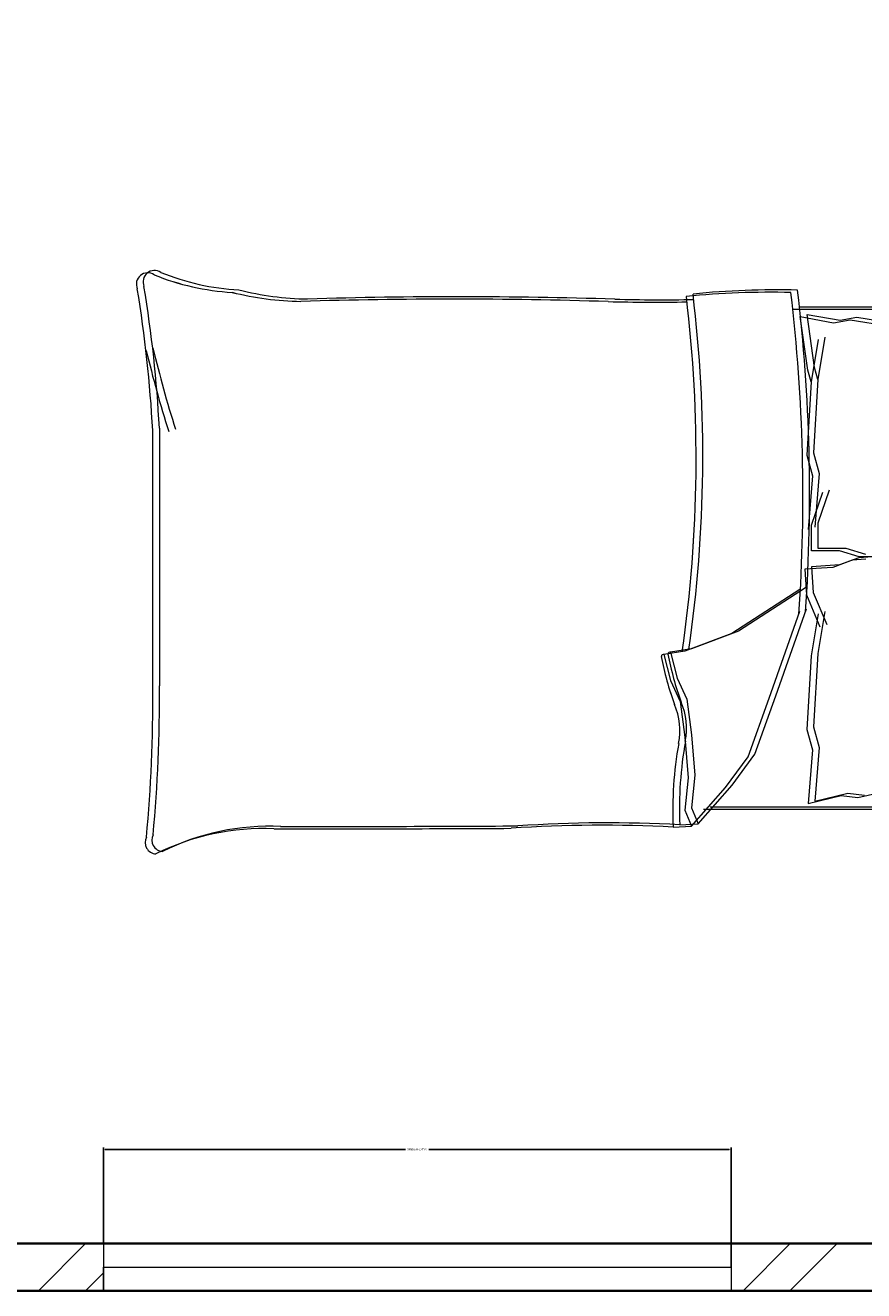
# Model space of a CAD drawing. Units: inches. Extents: x 2120 to 4013, y 1390 to 3019.
# Tile 11 of 59: x 2537 to 2617, y 1582 to 1702. Entities that reach past the tile are written whole.
import ezdxf

# ---------------------------------------------------------------- set-up
doc = ezdxf.new("R2010")
doc.units = ezdxf.units.IN
for name, color, linetype, lineweight in [('A-ANNO-DIMS', 2, 'Continuous', 18), ('A-FURN', 8, 'Continuous', 13), ('A-GLAZ', 4, 'Continuous', 18), ('A-WALL', 7, 'Continuous', 35), ('A-WALL-PATT', 252, 'Continuous', 13)]:
    doc.layers.add(name, color=color, linetype=linetype, lineweight=lineweight)
doc.styles.get("Standard").update_dxf_attribs({"font": 'arial.ttf'})
doc.dimstyles.get("Standard").update_dxf_attribs({"dimtxt": 0.18, "dimasz": 0.18, "dimexe": 0.18, "dimexo": 0.0625, "dimgap": 0.09, "dimtad": 0, "dimtih": 1, "dimtoh": 1, "dimdec": 4, "dimzin": 0, "dimdsep": 46, "dimtxsty": 'Standard', "dimcen": 0.09, "dimadec": 0, "dimazin": 0, "dimtfac": 1, "dimtdec": 4, "dimtofl": 0, "dimtmove": 0, "dimatfit": 3, "dimfxl": 1, "dimtolj": 1, "dimtzin": 0, "dimarcsym": 0})

# ---------------------------------------------------------------- blocks, each defined once
blk = doc.blocks.new('BED-DOUBLE-PLAN')
for p, q in [((3.48, 63.34), (3.48, 81.45)), ((51.27, 81.45), (51.27, 54.84)), ((3.7, 62.7), (3.7, 80.81)), ((51.5, 80.81), (51.5, 54.2)), ((50.34, 68.98), (49.54, 72.55)), ((4.47, 68.88), (5.05, 72.49)), ((4.7, 68.24), (5.28, 71.85)), ((27.36, 70.37), (27.44, 69.07)), ((27.37, 70.41), (27.37, 69.1)), ((27.14, 69.74), (26.56, 67.86)), ((27.37, 69.1), (26.79, 67.23)), ((27.44, 69.07), (28.13, 67.23)), ((27.58, 69.73), (27.67, 68.43)), ((49.92, 68.01), (50.11, 69.62)), ((50.15, 67.37), (50.34, 68.98)), ((4.76, 67.29), (4.47, 68.88)), ((4.99, 66.65), (4.7, 68.24)), ((26.56, 67.86), (26.56, 65.18)), ((27.67, 68.43), (28.36, 66.59)), ((50.7, 64.87), (49.92, 68.01)), ((4.19, 64.11), (4.76, 67.29)), ((4.41, 63.47), (4.99, 66.65)), ((26.79, 67.23), (26.79, 64.54)), ((28.13, 67.23), (28.3, 64.55)), ((28.36, 66.59), (28.53, 63.91)), ((50.93, 64.23), (50.15, 67.37)), ((6.38, 65.82), (10.42, 65.15)), ((24.1, 65.18), (20.96, 66.27)), ((24.33, 64.54), (21.19, 65.63)), ((30.75, 64.71), (33.82, 65.99)), ((30.98, 64.07), (34.05, 65.35)), ((32.57, 65.82), (36.6, 65.15)), ((9.28, 64.83), (4.19, 64.11)), ((9.51, 64.19), (4.41, 63.47)), ((6.61, 65.18), (10.64, 64.51)), ((10.42, 65.15), (9.28, 64.83)), ((10.64, 64.51), (9.51, 64.19)), ((10.42, 65.15), (17.43, 64.72)), ((10.64, 64.51), (17.65, 64.08)), ((17.43, 64.72), (19.39, 65.28)), ((17.65, 64.08), (19.61, 64.64)), ((19.39, 65.28), (24.52, 64.87)), ((19.61, 64.64), (24.75, 64.23)), ((26.56, 65.18), (24.1, 65.18)), ((26.79, 64.54), (24.33, 64.54)), ((28.3, 64.55), (30.75, 64.71)), ((32.79, 65.18), (36.83, 64.51)), ((36.6, 65.15), (43.61, 64.72)), ((36.83, 64.51), (43.84, 64.08)), ((43.61, 64.72), (45.57, 65.28)), ((43.84, 64.08), (45.8, 64.64)), ((45.57, 65.28), (50.7, 64.87)), ((45.8, 64.64), (50.93, 64.23)), ((28.53, 63.91), (30.98, 64.07)), ((30.26, 64.06), (34.45, 57.57)), ((30.49, 63.42), (34.68, 56.93)), ((40.65, 61.13), (32.31, 64.06)), ((40.87, 60.49), (32.54, 63.42)), ((46.22, 59.12), (40.65, 61.13)), ((46.45, 58.48), (40.87, 60.49)), ((49.16, 56.95), (46.22, 59.12)), ((49.39, 56.31), (46.45, 58.48)), ((34.45, 57.57), (36.15, 53.08)), ((34.68, 56.93), (36.38, 52.44)), ((52.87, 53.7), (49.16, 56.95)), ((53.1, 53.06), (49.39, 56.31)), ((44.36, 53.08), (48.23, 53.39)), ((48.23, 53.39), (51.33, 53.08)), ((51.33, 53.08), (52.87, 53.7)), ((52.95, 51.96), (52.87, 53.7, 3.87)), ((36.15, 53.08), (36.46, 51.07)), ((36.38, 52.44), (36.69, 50.43)), ((38.94, 51.69), (40.96, 52.62)), ((40.96, 52.62), (44.36, 53.08)), ((41.18, 51.98), (44.59, 52.44)), ((44.59, 52.44), (48.46, 52.75)), ((48.46, 52.75), (51.56, 52.44)), ((51.56, 52.44), (53.1, 53.06)), ((53.18, 51.32), (53.1, 53.06, 3.87)), ((36.46, 51.07), (38.94, 51.69)), ((36.69, 50.43), (39.17, 51.05)), ((39.17, 51.05), (41.18, 51.98)), ((15.06, 2.2), (39.68, 2.2)), ((15.29, 1.56), (39.91, 1.56))]:
    blk.add_line(p, q)
for centre, radius, start, end in [((21.36, -100.61), 164.97, 86.0865, 96.7821), ((85.16, 61.35), 83.31, 178.7218, 185.604), ((21.59, -101.25), 164.97, 86.0865, 96.7821), ((85.39, 60.71), 83.31, 178.7218, 185.604), ((17.76, -74.87), 129.02, 81.7845, 96.9006), ((17.99, -75.51), 129.02, 81.7845, 96.9006), ((-167.31, 50.27), 170.11, 358.4762, 1.0082), ((-167.08, 49.63), 170.11, 358.4762, 1.0082), ((31.16, 79.96), 29.65, 280.6617, 289.8806), ((43.74, 46.38), 6.22, 78.6608, 113.7384), ((51.33, 88.1), 36.18, 259.8763, 272.5657), ((36.64, 51.01), 0.185, 160.2464, 271.1377), ((31.38, 79.32), 29.65, 280.6617, 289.8806), ((43.97, 45.74), 6.22, 78.6608, 113.7384), ((51.56, 87.46), 36.18, 259.8763, 272.5657), ((182.27, 45.13), 129.5, 176.9791, 183.8365), ((182.5, 44.49), 129.5, 176.9791, 183.8365), ((36.87, 50.37), 0.185, 160.2464, 271.1377), ((484.82, 30.83), 482.31, 178.2277, 181.7185), ((485.05, 30.19), 482.31, 178.2277, 181.7185), ((-4508.74, 13.62), 4561.86, 0.00217, 0.28689), ((-4508.51, 12.99), 4561.86, 0.00217, 0.28689), ((-26.9, 16.93), 29.63, 346.0648, 358.9113), ((-26.67, 16.29), 29.63, 346.0648, 358.9113), ((76.16, 12.78), 23.07, 177.4714, 206.4681), ((76.39, 12.14), 23.07, 177.4714, 206.4681), ((-21.66, 11.17), 23.56, 337.9751, 356.652), ((-21.43, 10.53), 23.56, 337.9751, 356.652), ((-17.22, 105.16), 106.46, 283.3832, 287.7053), ((-16.99, 104.52), 106.46, 283.3832, 287.7053), ((54.41, 2.58), 1.1, 242.6588, 356.02), ((1.09, 1.73), 1.09, 146.1736, 293.4781), ((1.32, 1.09), 1.09, 146.1736, 293.4781), ((21.43, -119.39), 121.76, 92.9958, 99.4091), ((21.66, -120.03), 121.76, 92.9958, 99.4091), ((41.15, -130.83), 133.04, 84.4998, 90.6351), ((41.38, -131.47), 133.04, 84.4998, 90.6351), ((54.64, 1.94), 1.1, 242.6588, 356.02)]:
    blk.add_arc(centre, radius, start, end)
blk = doc.blocks.new('WIN-PLAN-60IN-05')
for p, q in [((0, 4.5), (0, 0)), ((60, 2.25), (60, 4.5)), ((60, 4.5), (60, 4.5)), ((60, 4.5), (60, 0)), ((0, 0), (0, 2.25)), ((0, 2.25), (60, 2.25))]:
    blk.add_line(p, q)
blk = doc.blocks.new('*D191')
at = {"layer": 'A-ANNO-DIMS', "color": 0, "lineweight": -2, "transparency": 16777216}
for p, q in [((2544.14, 1586.09), (2544.14, 1595.21)), ((2544.32, 1595.03), (2573.02, 1595.03)), ((2603.96, 1595.03), (2575.25, 1595.03)), ((2604.14, 1586.09), (2604.14, 1595.21))]:
    blk.add_line(p, q, dxfattribs=at)
at = {"layer": 'A-ANNO-DIMS', "color": 0, "transparency": 16777216}
for points in [[(2544.32, 1595.06), (2544.32, 1595), (2544.14, 1595.03)], [(2603.96, 1595.06), (2603.96, 1595), (2604.14, 1595.03)]]:
    blk.add_solid(points, dxfattribs=at)
at = {"layer": 'Defpoints', "color": 0, "transparency": 16777216}
for p in [(2604.14, 1595.03), (2544.14, 1586.03), (2604.14, 1586.03)]:
    blk.add_point(p, dxfattribs=at)
at = {"layer": 'A-ANNO-DIMS', "color": 0, "transparency": 16777216, "insert": (2574.14, 1595.03), "char_height": 0.18, "attachment_point": 5}
blk.add_mtext('\\A1;WINDOW 60 TYP.', dxfattribs=at)
blk = doc.blocks.new('*D192')
at = {"layer": 'A-ANNO-DIMS', "color": 0, "lineweight": -2, "transparency": 16777216}
for p, q in [((2544.07, 1586.03), (2534.96, 1586.03)), ((2535.14, 1585.85), (2535.14, 1583.96)), ((2535.14, 1581.71), (2535.14, 1583.6)), ((2544.07, 1581.53), (2534.96, 1581.53))]:
    blk.add_line(p, q, dxfattribs=at)
at = {"layer": 'A-ANNO-DIMS', "color": 0, "transparency": 16777216}
for points in [[(2535.11, 1585.85), (2535.17, 1585.85), (2535.14, 1586.03)], [(2535.11, 1581.71), (2535.17, 1581.71), (2535.14, 1581.53)]]:
    blk.add_solid(points, dxfattribs=at)
at = {"layer": 'Defpoints', "color": 0, "transparency": 16777216}
for p in [(2535.14, 1586.03), (2544.14, 1586.03), (2544.14, 1581.53)]:
    blk.add_point(p, dxfattribs=at)
at = {"layer": 'A-ANNO-DIMS', "color": 0, "transparency": 16777216, "insert": (2535.14, 1583.78), "char_height": 0.18, "attachment_point": 5}
blk.add_mtext('\\A1;5 TYP.', dxfattribs=at)

msp = doc.modelspace()

# ---------------------------------------------------------------- hatches: boundary and pattern name
at = {"layer": 'A-WALL-PATT'}
h = msp.add_hatch(dxfattribs=at)
h.set_pattern_fill('ANSI32', color=256)
h.paths.add_polyline_path([(2271.7331, 2343.531), (2283.3788, 2343.531), (2283.3788, 2348.031), (2283.3788, 2352.5306), (2262.7331, 2352.5306), (2262.7331, 2182.638), (2267.2331, 2182.638), (2271.7331, 2182.638), (2271.7331, 2219.031), (2391.7331, 2219.031), (2391.7331, 2214.189), (2393.9831, 2214.189), (2396.2331, 2214.189), (2396.2331, 2219.031), (2420.2331, 2219.031), (2420.2331, 2225.7535), (2417.2197, 2225.7535), (2415.7331, 2225.7535), (2415.7331, 2223.5306), (2271.7331, 2223.5306)])
h.paths.add_polyline_path([(2380.0942, 2352.5306), (2343.3788, 2352.5306), (2343.3788, 2343.531), (2363.2331, 2343.531), (2363.2331, 2288.8489), (2365.4831, 2288.8489), (2367.7331, 2288.8489), (2367.7331, 2343.531), (2380.0942, 2343.531)], flags=17)
h.paths.add_polyline_path([(2432.4339, 2352.5306), (2404.0943, 2352.5306), (2404.0943, 2343.531), (2415.7331, 2343.531), (2415.7331, 2264.0306), (2367.7331, 2264.0306), (2367.7331, 2266.4872), (2363.2331, 2266.4872), (2363.2331, 2259.531), (2367.7331, 2259.531), (2415.7331, 2259.531), (2415.7331, 2255.0658), (2420.2331, 2255.0658), (2420.2331, 2259.531), (2424.5717, 2259.531), (2424.5717, 2261.781), (2424.5717, 2264.0306), (2420.2331, 2264.0306), (2420.2331, 2343.531), (2432.4339, 2343.531)])
h.paths.add_polyline_path([(2508.9115, 2352.5306), (2456.4339, 2352.5306), (2456.4339, 2343.531), (2468.2331, 2343.531), (2468.2331, 2264.0306), (2448.0487, 2264.0306), (2448.0487, 2259.531), (2468.2331, 2259.531), (2468.2331, 2255.5496), (2472.7331, 2255.5496), (2472.7331, 2343.531), (2508.9115, 2343.531)])
h.paths.add_polyline_path([(2637.7331, 2352.5306), (2544.9116, 2352.5306), (2544.9116, 2343.531), (2589.7331, 2343.531), (2633.2331, 2343.531), (2637.7331, 2343.531)])
h.paths.add_polyline_path([(2594.2331, 2343.5306), (2589.7331, 2343.5306), (2589.7331, 2259.5306), (2589.7331, 2252.4915), (2591.9831, 2252.4915), (2594.2331, 2252.4915)])
h.paths.add_polyline_path([(2637.7331, 2223.5306), (2594.2331, 2223.5306), (2594.2331, 2230.1988), (2591.9831, 2230.1988), (2589.7331, 2230.1988), (2589.7331, 2223.5306), (2472.7331, 2223.5306), (2468.2331, 2223.5306), (2468.2331, 2219.031), (2628.7331, 2219.031), (2628.7331, 2138.031), (2637.7331, 2138.031)])
h.paths.add_polyline_path([(3822.6535, 2458.4402), (3874.9468, 2458.4402), (3874.9468, 2476.9866), (3822.6535, 2476.9866)], flags=9)
h.paths.add_polyline_path([(3834.6921, 2781.8174), (3935.9206, 2781.8174), (3935.9206, 2800.3638), (3834.6921, 2800.3638)], flags=9)
h.paths.add_polyline_path([(3832.2843, 2837.9683), (3884.5776, 2837.9683), (3884.5776, 2856.5146), (3832.2843, 2856.5146)], flags=9)
h.paths.add_polyline_path([(3830.9388, 2861.4782), (3956.8958, 2861.4782), (3956.8958, 2880.0245), (3830.9388, 2880.0245)], flags=9)
h.paths.add_polyline_path([(3870.6966, 2352.5752), (3887.9272, 2352.5752), (3887.9272, 2377.3037), (3870.6966, 2377.3037)], flags=9)
h.paths.add_polyline_path([(3289.2701, 2413.161), (3435.2223, 2413.161), (3435.2223, 2450.2538), (3289.2701, 2450.2538)], flags=9)
h.paths.add_polyline_path([(2487.6944, 2414.3601), (2637.8335, 2414.3601), (2637.8335, 2451.4528), (2487.6944, 2451.4528)], flags=9)
h.paths.add_polyline_path([(2567.3724, 1457.9199), (2815.296, 1457.9199), (2815.296, 1495.0127), (2567.3724, 1495.0127)], flags=9)
h.paths.add_polyline_path([(2655.3825, 2093.2363), (2685.9555, 2093.2363), (2685.9555, 2111.8937), (2655.3825, 2111.8937)], flags=9)
h.paths.add_polyline_path([(2543.9218, 1550.6671), (2587.8406, 1550.6671), (2587.8406, 1569.3244), (2543.9218, 1569.3244)], flags=9)
h.paths.add_polyline_path([(2905.1384, 1543.8113), (2949.0572, 1543.8113), (2949.0572, 1562.4686), (2905.1384, 1562.4686)], flags=9)
h.paths.add_polyline_path([(2736.4118, 1702.4736), (2784.2153, 1702.4736), (2784.2153, 1721.1309), (2736.4118, 1721.1309)], flags=9)
h.paths.add_polyline_path([(2912.8666, 1710.4168), (2951.707, 1710.4168), (2951.707, 1729.0741), (2912.8666, 1729.0741)], flags=9)
h.paths.add_polyline_path([(2923.5785, 1763.5038), (2959.7279, 1763.5038), (2959.7279, 1782.1611), (2923.5785, 1782.1611)], flags=9)
h.paths.add_polyline_path([(2925.2114, 1809.6137), (2967.1861, 1809.6137), (2967.1861, 1828.271), (2925.2114, 1828.271)], flags=9)
h.paths.add_polyline_path([(2996.2711, 1878.9003), (2996.2711, 1913.109), (2977.6138, 1913.109), (2977.6138, 1878.9003)], flags=9)
h.paths.add_polyline_path([(2883.0859, 1895.7192), (2927.1855, 1895.7192), (2927.1855, 1914.3766), (2883.0859, 1914.3766)], flags=9)
h.paths.add_polyline_path([(2787.3924, 1810.8013), (2841.0213, 1810.8013), (2841.0213, 1829.4587), (2787.3924, 1829.4587)], flags=9)
h.paths.add_polyline_path([(2775.6399, 2101.7395), (2829.2689, 2101.7395), (2829.2689, 2120.3968), (2775.6399, 2120.3968)], flags=9)
h.paths.add_polyline_path([(2913.0263, 2075.817), (2951.8667, 2075.817), (2951.8667, 2094.4744), (2913.0263, 2094.4744)], flags=9)
h.paths.add_polyline_path([(2929.966, 2133.3669), (2966.1154, 2133.3669), (2966.1154, 2152.0243), (2929.966, 2152.0243)], flags=9)
h.paths.add_polyline_path([(2932.7502, 2182.6088), (2968.8996, 2182.6088), (2968.8996, 2201.2662), (2932.7502, 2201.2662)], flags=9)
h.paths.add_polyline_path([(2996.0681, 2266.3173), (2996.0681, 2300.5261), (2977.4108, 2300.5261), (2977.4108, 2266.3173)], flags=9)
h.paths.add_polyline_path([(2885.1039, 2279.2186), (2929.2035, 2279.2186), (2929.2035, 2297.8759), (2885.1039, 2297.8759)], flags=9)
h.paths.add_polyline_path([(2735.7042, 2218.3197), (2783.5078, 2218.3197), (2783.5078, 2236.9771), (2735.7042, 2236.9771)], flags=9)
h.paths.add_polyline_path([(2635.6049, 2044.0085), (2648.9678, 2044.0085), (2648.9678, 2054.312), (2635.6049, 2054.312)], flags=9)
h.paths.add_polyline_path([(2714.0148, 1923.0473), (2727.3777, 1923.0473), (2727.3777, 1933.3508), (2714.0148, 1933.3508)], flags=9)
h.paths.add_polyline_path([(2709.0345, 1988.1628), (2722.3974, 1988.1628), (2722.3974, 1998.4663), (2709.0345, 1998.4663)], flags=9)
h.paths.add_polyline_path([(2592.8935, 1962.1763), (2606.2564, 1962.1763), (2606.2564, 1972.4799), (2592.8935, 1972.4799)], flags=9)
h.paths.add_polyline_path([(2618.3996, 1985.9724), (2644.1942, 1985.9724), (2644.1942, 1996.2759), (2618.3996, 1996.2759)], flags=9)
h.paths.add_polyline_path([(2601.279, 1920.5869), (2614.6419, 1920.5869), (2614.6419, 1930.8904), (2601.279, 1930.8904)], flags=9)
h.paths.add_polyline_path([(2692.3278, 1932.7645), (2704.5311, 1932.7645), (2704.5311, 1943.0681), (2692.3278, 1943.0681)], flags=9)
h.paths.add_polyline_path([(2311.122, 1672.7318), (2355.0408, 1672.7318), (2355.0408, 1691.3892), (2311.122, 1691.3892)], flags=9)
h.paths.add_polyline_path([(2456.2551, 1632.3198), (2492.4796, 1632.3198), (2492.4796, 1650.9772), (2456.2551, 1650.9772)], flags=9)
h.paths.add_polyline_path([(2401.0766, 1631.4793), (2437.301, 1631.4793), (2437.301, 1650.1367), (2401.0766, 1650.1367)], flags=9)
h.paths.add_polyline_path([(2546.7054, 1700.9235), (2594.509, 1700.9235), (2594.509, 1719.5809), (2546.7054, 1719.5809)], flags=9)
h.paths.add_polyline_path([(2445.4866, 1766.9937), (2497.5261, 1766.9937), (2497.5261, 1785.651), (2445.4866, 1785.651)], flags=9)
h.paths.add_polyline_path([(2287.9992, 1739.7675), (2326.8396, 1739.7675), (2326.8396, 1758.4248), (2287.9992, 1758.4248)], flags=9)
h.paths.add_polyline_path([(2458.5279, 1924.7607), (2510.5675, 1924.7607), (2510.5675, 1943.4181), (2458.5279, 1943.4181)], flags=9)
h.paths.add_polyline_path([(2309.2811, 1902.7642), (2345.4305, 1902.7642), (2345.4305, 1921.4215), (2309.2811, 1921.4215)], flags=9)
h.paths.add_polyline_path([(2490.7554, 2018.9392), (2530.7896, 2018.9392), (2530.7896, 2037.5965), (2490.7554, 2037.5965)], flags=9)
h.paths.add_polyline_path([(2402.143, 2024.7393), (2438.5414, 2024.7393), (2438.5414, 2043.3966), (2402.143, 2043.3966)], flags=9)
h.paths.add_polyline_path([(2287.856, 1931.7926), (2326.6964, 1931.7926), (2326.6964, 1950.4499), (2287.856, 1950.4499)], flags=9)
h.paths.add_polyline_path([(2281.7979, 2193.5771), (2320.6383, 2193.5771), (2320.6383, 2212.2344), (2281.7979, 2212.2344)], flags=25)
h.paths.add_polyline_path([(2484.0754, 2093.892), (2536.115, 2093.892), (2536.115, 2112.5494), (2484.0754, 2112.5494)], flags=9)
h.paths.add_polyline_path([(2624.7948, 2281.8639), (2624.7948, 2311.4137), (2606.1375, 2311.4137), (2606.1375, 2281.8639)], flags=9)
h.paths.add_polyline_path([(2507.5036, 2290.3639), (2541.934, 2290.3639), (2541.934, 2309.0212), (2507.5036, 2309.0212)], flags=9)
h.paths.add_polyline_path([(2423.1076, 2285.2202), (2459.332, 2285.2202), (2459.332, 2303.8776), (2423.1076, 2303.8776)], flags=9)
h.paths.add_polyline_path([(2374.5467, 2289.6272), (2410.7711, 2289.6272), (2410.7711, 2308.2846), (2374.5467, 2308.2846)], flags=25)
h.paths.add_polyline_path([(2277.4907, 2227.5651), (2316.3311, 2227.5651), (2316.3311, 2246.2224), (2277.4907, 2246.2224)], flags=25)
h.paths.add_polyline_path([(2655.3825, 2093.2367), (2685.9555, 2093.2367), (2685.9555, 2111.894), (2655.3825, 2111.894)], flags=9)
h.paths.add_polyline_path([(2543.9217, 1550.6674), (2587.8406, 1550.6674), (2587.8406, 1569.3247), (2543.9217, 1569.3247)], flags=9)
h.paths.add_polyline_path([(2905.1384, 1543.8116), (2949.0572, 1543.8116), (2949.0572, 1562.4689), (2905.1384, 1562.4689)], flags=9)
h.paths.add_polyline_path([(2736.4118, 1702.4739), (2784.2153, 1702.4739), (2784.2153, 1721.1312), (2736.4118, 1721.1312)], flags=9)
h.paths.add_polyline_path([(2912.8666, 1710.4171), (2951.707, 1710.4171), (2951.707, 1729.0744), (2912.8666, 1729.0744)], flags=9)
h.paths.add_polyline_path([(2923.5785, 1763.5041), (2959.7279, 1763.5041), (2959.7279, 1782.1614), (2923.5785, 1782.1614)], flags=9)
h.paths.add_polyline_path([(2925.2114, 1809.614), (2967.1861, 1809.614), (2967.1861, 1828.2713), (2925.2114, 1828.2713)], flags=9)
h.paths.add_polyline_path([(2996.2711, 1878.9006), (2996.2711, 1913.1094), (2977.6137, 1913.1094), (2977.6137, 1878.9006)], flags=9)
h.paths.add_polyline_path([(2883.0859, 1895.7195), (2927.1855, 1895.7195), (2927.1855, 1914.3769), (2883.0859, 1914.3769)], flags=9)
h.paths.add_polyline_path([(2787.3924, 1810.8016), (2841.0213, 1810.8016), (2841.0213, 1829.459), (2787.3924, 1829.459)], flags=9)
h.paths.add_polyline_path([(2775.6399, 2101.7398), (2829.2688, 2101.7398), (2829.2688, 2120.3971), (2775.6399, 2120.3971)], flags=9)
h.paths.add_polyline_path([(2913.0263, 2075.8173), (2951.8667, 2075.8173), (2951.8667, 2094.4747), (2913.0263, 2094.4747)], flags=9)
h.paths.add_polyline_path([(2929.966, 2133.3672), (2966.1154, 2133.3672), (2966.1154, 2152.0246), (2929.966, 2152.0246)], flags=9)
h.paths.add_polyline_path([(2932.7502, 2182.6091), (2968.8996, 2182.6091), (2968.8996, 2201.2665), (2932.7502, 2201.2665)], flags=9)
h.paths.add_polyline_path([(2996.0681, 2266.3176), (2996.0681, 2300.5264), (2977.4108, 2300.5264), (2977.4108, 2266.3176)], flags=9)
h.paths.add_polyline_path([(2885.1039, 2279.2189), (2929.2035, 2279.2189), (2929.2035, 2297.8762), (2885.1039, 2297.8762)], flags=9)
h.paths.add_polyline_path([(2735.7042, 2218.32), (2783.5078, 2218.32), (2783.5078, 2236.9774), (2735.7042, 2236.9774)], flags=9)
h.paths.add_polyline_path([(2635.6048, 2044.0088), (2648.9677, 2044.0088), (2648.9677, 2054.3123), (2635.6048, 2054.3123)], flags=9)
h.paths.add_polyline_path([(2714.0148, 1923.0476), (2727.3777, 1923.0476), (2727.3777, 1933.3511), (2714.0148, 1933.3511)], flags=9)
h.paths.add_polyline_path([(2709.0345, 1988.1631), (2722.3974, 1988.1631), (2722.3974, 1998.4666), (2709.0345, 1998.4666)], flags=9)
h.paths.add_polyline_path([(2592.8935, 1962.1766), (2606.2564, 1962.1766), (2606.2564, 1972.4802), (2592.8935, 1972.4802)], flags=9)
h.paths.add_polyline_path([(2618.3995, 1985.9727), (2644.1942, 1985.9727), (2644.1942, 1996.2762), (2618.3995, 1996.2762)], flags=9)
h.paths.add_polyline_path([(2601.279, 1920.5872), (2614.6419, 1920.5872), (2614.6419, 1930.8908), (2601.279, 1930.8908)], flags=9)
h.paths.add_polyline_path([(2692.3278, 1932.7648), (2704.5311, 1932.7648), (2704.5311, 1943.0684), (2692.3278, 1943.0684)], flags=9)
h.paths.add_polyline_path([(2311.122, 1672.7321), (2355.0408, 1672.7321), (2355.0408, 1691.3895), (2311.122, 1691.3895)], flags=9)
h.paths.add_polyline_path([(2456.2551, 1632.3201), (2492.4795, 1632.3201), (2492.4795, 1650.9775), (2456.2551, 1650.9775)], flags=9)
h.paths.add_polyline_path([(2401.0766, 1631.4796), (2437.301, 1631.4796), (2437.301, 1650.137), (2401.0766, 1650.137)], flags=9)
h.paths.add_polyline_path([(2546.7054, 1700.9238), (2594.509, 1700.9238), (2594.509, 1719.5812), (2546.7054, 1719.5812)], flags=9)
h.paths.add_polyline_path([(2445.4866, 1766.994), (2497.5261, 1766.994), (2497.5261, 1785.6513), (2445.4866, 1785.6513)], flags=9)
h.paths.add_polyline_path([(2287.9992, 1739.7678), (2326.8396, 1739.7678), (2326.8396, 1758.4251), (2287.9992, 1758.4251)], flags=9)
h.paths.add_polyline_path([(2458.5279, 1924.7611), (2510.5675, 1924.7611), (2510.5675, 1943.4184), (2458.5279, 1943.4184)], flags=9)
h.paths.add_polyline_path([(2309.2811, 1902.7645), (2345.4305, 1902.7645), (2345.4305, 1921.4218), (2309.2811, 1921.4218)], flags=9)
h.paths.add_polyline_path([(2490.7554, 2018.9395), (2530.7895, 2018.9395), (2530.7895, 2037.5968), (2490.7554, 2037.5968)], flags=9)
h.paths.add_polyline_path([(2402.143, 2024.7396), (2438.5413, 2024.7396), (2438.5413, 2043.3969), (2402.143, 2043.3969)], flags=9)
h.paths.add_polyline_path([(2287.856, 1931.7929), (2326.6964, 1931.7929), (2326.6964, 1950.4502), (2287.856, 1950.4502)], flags=9)
h.paths.add_polyline_path([(2281.7979, 2193.5774), (2320.6383, 2193.5774), (2320.6383, 2212.2347), (2281.7979, 2212.2347)], flags=25)
h.paths.add_polyline_path([(2484.0754, 2093.8924), (2536.115, 2093.8924), (2536.115, 2112.5497), (2484.0754, 2112.5497)], flags=9)
h.paths.add_polyline_path([(2624.7948, 2281.8642), (2624.7948, 2311.414), (2606.1374, 2311.414), (2606.1374, 2281.8642)], flags=9)
h.paths.add_polyline_path([(2507.5035, 2290.3642), (2541.934, 2290.3642), (2541.934, 2309.0215), (2507.5035, 2309.0215)], flags=9)
h.paths.add_polyline_path([(2423.1075, 2285.2205), (2459.332, 2285.2205), (2459.332, 2303.8779), (2423.1075, 2303.8779)], flags=9)
h.paths.add_polyline_path([(2374.5467, 2289.6275), (2410.7711, 2289.6275), (2410.7711, 2308.2849), (2374.5467, 2308.2849)], flags=25)
h.paths.add_polyline_path([(2277.4907, 2227.5654), (2316.3311, 2227.5654), (2316.3311, 2246.2227), (2277.4907, 2246.2227)], flags=25)
h = msp.add_hatch(dxfattribs=at)
h.set_pattern_fill('ANSI32', color=256)
h.paths.add_polyline_path([(2271.7331, 1980.389), (2262.7331, 1980.389), (2262.7331, 1912.8434), (2267.2331, 1912.8434), (2271.7331, 1912.8434), (2271.7331, 1922.531), (2351.2331, 1922.531), (2351.2331, 1901.4728), (2355.7331, 1901.4728), (2355.7331, 1922.531), (2357.9815, 1922.531), (2357.9815, 1926.5306), (2271.7331, 1926.5306)])
h.paths.add_polyline_path([(2589.2331, 1949.1622), (2584.7331, 1949.1622), (2580.2331, 1949.1622), (2580.2331, 1874.5306), (2355.7331, 1874.5306), (2355.7331, 1880.1922), (2351.2331, 1880.1922), (2351.2331, 1874.5306), (2271.7331, 1874.5306), (2271.7331, 1888.8431), (2262.7331, 1888.8431), (2262.7331, 1842.2909), (2267.2331, 1842.2909), (2271.7331, 1842.2909), (2271.7331, 1865.531), (2415.7331, 1865.531), (2415.7331, 1779.7286), (2420.2331, 1779.7286), (2420.2331, 1865.531), (2589.2331, 1865.531)])
h.paths.add_polyline_path([(2271.7331, 1782.2906), (2262.7331, 1782.2906), (2262.7331, 1711.4639), (2267.2331, 1711.4639), (2271.7331, 1711.4639), (2271.7331, 1738.031), (2420.2331, 1738.031), (2420.2331, 1742.531), (2420.2331, 1747.3376), (2417.9831, 1747.3376), (2415.7331, 1747.3376), (2415.7331, 1742.5306), (2271.7331, 1742.5306)])
h.paths.add_polyline_path([(2271.7331, 1627.031), (2362.3957, 1627.031), (2362.3957, 1629.281), (2362.3957, 1631.5306), (2271.7331, 1631.5306), (2271.7331, 1675.4636), (2262.7331, 1675.4636), (2262.7331, 1581.531), (2405.3032, 1581.531), (2405.3032, 1586.031), (2405.3032, 1590.5306), (2396.2331, 1590.5306), (2396.2331, 1691.4513), (2418.7206, 1691.4513), (2418.7206, 1695.951), (2396.2331, 1695.951), (2391.7331, 1695.951), (2391.7331, 1631.5306), (2386.7425, 1631.5306), (2386.7425, 1629.2806), (2386.7425, 1627.031), (2391.7331, 1627.031), (2391.7331, 1586.1709), (2271.7331, 1586.1709)])
h.paths.add_polyline_path([(2459.6703, 1590.5306), (2429.3032, 1590.5306), (2429.3032, 1581.531), (2459.6703, 1581.531), (2459.6703, 1586.031)])
h.paths.add_polyline_path([(2501.2331, 1590.531), (2501.2331, 1665.0195), (2498.9831, 1665.0195), (2496.7331, 1665.0195), (2496.7331, 1590.5306), (2483.8201, 1590.5306), (2483.8201, 1590.1579), (2483.6704, 1590.1579), (2483.6704, 1581.531), (2505.0196, 1581.531), (2505.0196, 1583.781), (2505.0196, 1586.0306), (2501.2331, 1586.0306)])
h.paths.add_polyline_path([(2544.1361, 1583.781), (2544.1361, 1586.0306), (2527.1368, 1586.0306), (2527.1368, 1583.7806), (2527.1368, 1581.531), (2544.1361, 1581.531)])
h.paths.add_polyline_path([(3822.6535, 2458.4402), (3874.9468, 2458.4402), (3874.9468, 2476.9866), (3822.6535, 2476.9866)], flags=9)
h.paths.add_polyline_path([(3834.6921, 2781.8174), (3935.9206, 2781.8174), (3935.9206, 2800.3638), (3834.6921, 2800.3638)], flags=9)
h.paths.add_polyline_path([(3832.2843, 2837.9683), (3884.5776, 2837.9683), (3884.5776, 2856.5146), (3832.2843, 2856.5146)], flags=9)
h.paths.add_polyline_path([(3830.9388, 2861.4782), (3956.8958, 2861.4782), (3956.8958, 2880.0245), (3830.9388, 2880.0245)], flags=9)
h.paths.add_polyline_path([(3870.6966, 2352.5752), (3887.9272, 2352.5752), (3887.9272, 2377.3037), (3870.6966, 2377.3037)], flags=9)
h.paths.add_polyline_path([(3289.2701, 2413.161), (3435.2223, 2413.161), (3435.2223, 2450.2538), (3289.2701, 2450.2538)], flags=9)
h.paths.add_polyline_path([(2487.6944, 2414.3601), (2637.8335, 2414.3601), (2637.8335, 2451.4528), (2487.6944, 2451.4528)], flags=9)
h.paths.add_polyline_path([(2567.3724, 1457.9199), (2815.296, 1457.9199), (2815.296, 1495.0127), (2567.3724, 1495.0127)], flags=9)
h.paths.add_polyline_path([(2655.3825, 2093.2363), (2685.9555, 2093.2363), (2685.9555, 2111.8937), (2655.3825, 2111.8937)], flags=9)
h.paths.add_polyline_path([(2543.9218, 1550.6671), (2587.8406, 1550.6671), (2587.8406, 1569.3244), (2543.9218, 1569.3244)], flags=9)
h.paths.add_polyline_path([(2905.1384, 1543.8113), (2949.0572, 1543.8113), (2949.0572, 1562.4686), (2905.1384, 1562.4686)], flags=9)
h.paths.add_polyline_path([(2736.4118, 1702.4736), (2784.2153, 1702.4736), (2784.2153, 1721.1309), (2736.4118, 1721.1309)], flags=9)
h.paths.add_polyline_path([(2912.8666, 1710.4168), (2951.707, 1710.4168), (2951.707, 1729.0741), (2912.8666, 1729.0741)], flags=9)
h.paths.add_polyline_path([(2923.5785, 1763.5038), (2959.7279, 1763.5038), (2959.7279, 1782.1611), (2923.5785, 1782.1611)], flags=9)
h.paths.add_polyline_path([(2925.2114, 1809.6137), (2967.1861, 1809.6137), (2967.1861, 1828.271), (2925.2114, 1828.271)], flags=9)
h.paths.add_polyline_path([(2996.2711, 1878.9003), (2996.2711, 1913.109), (2977.6138, 1913.109), (2977.6138, 1878.9003)], flags=9)
h.paths.add_polyline_path([(2883.0859, 1895.7192), (2927.1855, 1895.7192), (2927.1855, 1914.3766), (2883.0859, 1914.3766)], flags=9)
h.paths.add_polyline_path([(2787.3924, 1810.8013), (2841.0213, 1810.8013), (2841.0213, 1829.4587), (2787.3924, 1829.4587)], flags=9)
h.paths.add_polyline_path([(2775.6399, 2101.7395), (2829.2689, 2101.7395), (2829.2689, 2120.3968), (2775.6399, 2120.3968)], flags=9)
h.paths.add_polyline_path([(2913.0263, 2075.817), (2951.8667, 2075.817), (2951.8667, 2094.4744), (2913.0263, 2094.4744)], flags=9)
h.paths.add_polyline_path([(2929.966, 2133.3669), (2966.1154, 2133.3669), (2966.1154, 2152.0243), (2929.966, 2152.0243)], flags=9)
h.paths.add_polyline_path([(2932.7502, 2182.6088), (2968.8996, 2182.6088), (2968.8996, 2201.2662), (2932.7502, 2201.2662)], flags=9)
h.paths.add_polyline_path([(2996.0681, 2266.3173), (2996.0681, 2300.5261), (2977.4108, 2300.5261), (2977.4108, 2266.3173)], flags=9)
h.paths.add_polyline_path([(2885.1039, 2279.2186), (2929.2035, 2279.2186), (2929.2035, 2297.8759), (2885.1039, 2297.8759)], flags=9)
h.paths.add_polyline_path([(2735.7042, 2218.3197), (2783.5078, 2218.3197), (2783.5078, 2236.9771), (2735.7042, 2236.9771)], flags=9)
h.paths.add_polyline_path([(2635.6049, 2044.0085), (2648.9678, 2044.0085), (2648.9678, 2054.312), (2635.6049, 2054.312)], flags=9)
h.paths.add_polyline_path([(2714.0148, 1923.0473), (2727.3777, 1923.0473), (2727.3777, 1933.3508), (2714.0148, 1933.3508)], flags=9)
h.paths.add_polyline_path([(2709.0345, 1988.1628), (2722.3974, 1988.1628), (2722.3974, 1998.4663), (2709.0345, 1998.4663)], flags=9)
h.paths.add_polyline_path([(2592.8935, 1962.1763), (2606.2564, 1962.1763), (2606.2564, 1972.4799), (2592.8935, 1972.4799)], flags=9)
h.paths.add_polyline_path([(2618.3996, 1985.9724), (2644.1942, 1985.9724), (2644.1942, 1996.2759), (2618.3996, 1996.2759)], flags=9)
h.paths.add_polyline_path([(2601.279, 1920.5869), (2614.6419, 1920.5869), (2614.6419, 1930.8904), (2601.279, 1930.8904)], flags=9)
h.paths.add_polyline_path([(2692.3278, 1932.7645), (2704.5311, 1932.7645), (2704.5311, 1943.0681), (2692.3278, 1943.0681)], flags=9)
h.paths.add_polyline_path([(2311.122, 1672.7318), (2355.0408, 1672.7318), (2355.0408, 1691.3892), (2311.122, 1691.3892)], flags=25)
h.paths.add_polyline_path([(2456.2551, 1632.3198), (2492.4796, 1632.3198), (2492.4796, 1650.9772), (2456.2551, 1650.9772)], flags=9)
h.paths.add_polyline_path([(2401.0766, 1631.4793), (2437.301, 1631.4793), (2437.301, 1650.1367), (2401.0766, 1650.1367)], flags=9)
h.paths.add_polyline_path([(2546.7054, 1700.9235), (2594.509, 1700.9235), (2594.509, 1719.5809), (2546.7054, 1719.5809)], flags=9)
h.paths.add_polyline_path([(2445.4866, 1766.9937), (2497.5261, 1766.9937), (2497.5261, 1785.651), (2445.4866, 1785.651)], flags=9)
h.paths.add_polyline_path([(2287.9992, 1739.7675), (2326.8396, 1739.7675), (2326.8396, 1758.4248), (2287.9992, 1758.4248)], flags=24)
h.paths.add_polyline_path([(2458.5279, 1924.7607), (2510.5675, 1924.7607), (2510.5675, 1943.4181), (2458.5279, 1943.4181)], flags=25)
h.paths.add_polyline_path([(2309.2811, 1902.7642), (2345.4305, 1902.7642), (2345.4305, 1921.4215), (2309.2811, 1921.4215)], flags=25)
h.paths.add_polyline_path([(2490.7554, 2018.9392), (2530.7896, 2018.9392), (2530.7896, 2037.5965), (2490.7554, 2037.5965)], flags=9)
h.paths.add_polyline_path([(2402.143, 2024.7393), (2438.5414, 2024.7393), (2438.5414, 2043.3966), (2402.143, 2043.3966)], flags=9)
h.paths.add_polyline_path([(2287.856, 1931.7926), (2326.6964, 1931.7926), (2326.6964, 1950.4499), (2287.856, 1950.4499)], flags=25)
h.paths.add_polyline_path([(2281.7979, 2193.5771), (2320.6383, 2193.5771), (2320.6383, 2212.2344), (2281.7979, 2212.2344)], flags=9)
h.paths.add_polyline_path([(2484.0754, 2093.892), (2536.115, 2093.892), (2536.115, 2112.5494), (2484.0754, 2112.5494)], flags=9)
h.paths.add_polyline_path([(2624.7948, 2281.8639), (2624.7948, 2311.4137), (2606.1375, 2311.4137), (2606.1375, 2281.8639)], flags=9)
h.paths.add_polyline_path([(2507.5036, 2290.3639), (2541.934, 2290.3639), (2541.934, 2309.0212), (2507.5036, 2309.0212)], flags=9)
h.paths.add_polyline_path([(2423.1076, 2285.2202), (2459.332, 2285.2202), (2459.332, 2303.8776), (2423.1076, 2303.8776)], flags=9)
h.paths.add_polyline_path([(2374.5467, 2289.6272), (2410.7711, 2289.6272), (2410.7711, 2308.2846), (2374.5467, 2308.2846)], flags=9)
h.paths.add_polyline_path([(2277.4907, 2227.5651), (2316.3311, 2227.5651), (2316.3311, 2246.2224), (2277.4907, 2246.2224)], flags=9)
h.paths.add_polyline_path([(2655.3825, 2093.2367), (2685.9555, 2093.2367), (2685.9555, 2111.894), (2655.3825, 2111.894)], flags=9)
h.paths.add_polyline_path([(2543.9217, 1550.6674), (2587.8406, 1550.6674), (2587.8406, 1569.3247), (2543.9217, 1569.3247)], flags=9)
h.paths.add_polyline_path([(2905.1384, 1543.8116), (2949.0572, 1543.8116), (2949.0572, 1562.4689), (2905.1384, 1562.4689)], flags=9)
h.paths.add_polyline_path([(2736.4118, 1702.4739), (2784.2153, 1702.4739), (2784.2153, 1721.1312), (2736.4118, 1721.1312)], flags=9)
h.paths.add_polyline_path([(2912.8666, 1710.4171), (2951.707, 1710.4171), (2951.707, 1729.0744), (2912.8666, 1729.0744)], flags=9)
h.paths.add_polyline_path([(2923.5785, 1763.5041), (2959.7279, 1763.5041), (2959.7279, 1782.1614), (2923.5785, 1782.1614)], flags=9)
h.paths.add_polyline_path([(2925.2114, 1809.614), (2967.1861, 1809.614), (2967.1861, 1828.2713), (2925.2114, 1828.2713)], flags=9)
h.paths.add_polyline_path([(2996.2711, 1878.9006), (2996.2711, 1913.1094), (2977.6137, 1913.1094), (2977.6137, 1878.9006)], flags=9)
h.paths.add_polyline_path([(2883.0859, 1895.7195), (2927.1855, 1895.7195), (2927.1855, 1914.3769), (2883.0859, 1914.3769)], flags=9)
h.paths.add_polyline_path([(2787.3924, 1810.8016), (2841.0213, 1810.8016), (2841.0213, 1829.459), (2787.3924, 1829.459)], flags=9)
h.paths.add_polyline_path([(2775.6399, 2101.7398), (2829.2688, 2101.7398), (2829.2688, 2120.3971), (2775.6399, 2120.3971)], flags=9)
h.paths.add_polyline_path([(2913.0263, 2075.8173), (2951.8667, 2075.8173), (2951.8667, 2094.4747), (2913.0263, 2094.4747)], flags=9)
h.paths.add_polyline_path([(2929.966, 2133.3672), (2966.1154, 2133.3672), (2966.1154, 2152.0246), (2929.966, 2152.0246)], flags=9)
h.paths.add_polyline_path([(2932.7502, 2182.6091), (2968.8996, 2182.6091), (2968.8996, 2201.2665), (2932.7502, 2201.2665)], flags=9)
h.paths.add_polyline_path([(2996.0681, 2266.3176), (2996.0681, 2300.5264), (2977.4108, 2300.5264), (2977.4108, 2266.3176)], flags=9)
h.paths.add_polyline_path([(2885.1039, 2279.2189), (2929.2035, 2279.2189), (2929.2035, 2297.8762), (2885.1039, 2297.8762)], flags=9)
h.paths.add_polyline_path([(2735.7042, 2218.32), (2783.5078, 2218.32), (2783.5078, 2236.9774), (2735.7042, 2236.9774)], flags=9)
h.paths.add_polyline_path([(2635.6048, 2044.0088), (2648.9677, 2044.0088), (2648.9677, 2054.3123), (2635.6048, 2054.3123)], flags=9)
h.paths.add_polyline_path([(2714.0148, 1923.0476), (2727.3777, 1923.0476), (2727.3777, 1933.3511), (2714.0148, 1933.3511)], flags=9)
h.paths.add_polyline_path([(2709.0345, 1988.1631), (2722.3974, 1988.1631), (2722.3974, 1998.4666), (2709.0345, 1998.4666)], flags=9)
h.paths.add_polyline_path([(2592.8935, 1962.1766), (2606.2564, 1962.1766), (2606.2564, 1972.4802), (2592.8935, 1972.4802)], flags=9)
h.paths.add_polyline_path([(2618.3995, 1985.9727), (2644.1942, 1985.9727), (2644.1942, 1996.2762), (2618.3995, 1996.2762)], flags=9)
h.paths.add_polyline_path([(2601.279, 1920.5872), (2614.6419, 1920.5872), (2614.6419, 1930.8908), (2601.279, 1930.8908)], flags=9)
h.paths.add_polyline_path([(2692.3278, 1932.7648), (2704.5311, 1932.7648), (2704.5311, 1943.0684), (2692.3278, 1943.0684)], flags=9)
h.paths.add_polyline_path([(2311.122, 1672.7321), (2355.0408, 1672.7321), (2355.0408, 1691.3895), (2311.122, 1691.3895)], flags=25)
h.paths.add_polyline_path([(2456.2551, 1632.3201), (2492.4795, 1632.3201), (2492.4795, 1650.9775), (2456.2551, 1650.9775)], flags=9)
h.paths.add_polyline_path([(2401.0766, 1631.4796), (2437.301, 1631.4796), (2437.301, 1650.137), (2401.0766, 1650.137)], flags=9)
h.paths.add_polyline_path([(2546.7054, 1700.9238), (2594.509, 1700.9238), (2594.509, 1719.5812), (2546.7054, 1719.5812)], flags=9)
h.paths.add_polyline_path([(2445.4866, 1766.994), (2497.5261, 1766.994), (2497.5261, 1785.6513), (2445.4866, 1785.6513)], flags=9)
h.paths.add_polyline_path([(2287.9992, 1739.7678), (2326.8396, 1739.7678), (2326.8396, 1758.4251), (2287.9992, 1758.4251)], flags=24)
h.paths.add_polyline_path([(2458.5279, 1924.7611), (2510.5675, 1924.7611), (2510.5675, 1943.4184), (2458.5279, 1943.4184)], flags=25)
h.paths.add_polyline_path([(2309.2811, 1902.7645), (2345.4305, 1902.7645), (2345.4305, 1921.4218), (2309.2811, 1921.4218)], flags=25)
h.paths.add_polyline_path([(2490.7554, 2018.9395), (2530.7895, 2018.9395), (2530.7895, 2037.5968), (2490.7554, 2037.5968)], flags=9)
h.paths.add_polyline_path([(2402.143, 2024.7396), (2438.5413, 2024.7396), (2438.5413, 2043.3969), (2402.143, 2043.3969)], flags=9)
h.paths.add_polyline_path([(2287.856, 1931.7929), (2326.6964, 1931.7929), (2326.6964, 1950.4502), (2287.856, 1950.4502)], flags=25)
h.paths.add_polyline_path([(2281.7979, 2193.5774), (2320.6383, 2193.5774), (2320.6383, 2212.2347), (2281.7979, 2212.2347)], flags=9)
h.paths.add_polyline_path([(2484.0754, 2093.8924), (2536.115, 2093.8924), (2536.115, 2112.5497), (2484.0754, 2112.5497)], flags=9)
h.paths.add_polyline_path([(2624.7948, 2281.8642), (2624.7948, 2311.414), (2606.1374, 2311.414), (2606.1374, 2281.8642)], flags=9)
h.paths.add_polyline_path([(2507.5035, 2290.3642), (2541.934, 2290.3642), (2541.934, 2309.0215), (2507.5035, 2309.0215)], flags=9)
h.paths.add_polyline_path([(2423.1075, 2285.2205), (2459.332, 2285.2205), (2459.332, 2303.8779), (2423.1075, 2303.8779)], flags=9)
h.paths.add_polyline_path([(2374.5467, 2289.6275), (2410.7711, 2289.6275), (2410.7711, 2308.2849), (2374.5467, 2308.2849)], flags=9)
h.paths.add_polyline_path([(2277.4907, 2227.5654), (2316.3311, 2227.5654), (2316.3311, 2246.2227), (2277.4907, 2246.2227)], flags=9)
h = msp.add_hatch(dxfattribs=at)
h.set_pattern_fill('ANSI32', color=256)
h.paths.add_polyline_path([(2271.7331, 2122.6377), (2262.7331, 2122.6377), (2262.7331, 2040.3893), (2267.2331, 2040.3893), (2271.7331, 2040.3893), (2271.7331, 2044.8856), (2271.7331, 2070.531), (2391.7331, 2070.531), (2391.7331, 1926.5306), (2388.3993, 1926.5306), (2388.3993, 1922.531), (2395.7331, 1922.531), (2395.7331, 1992.531), (2400.4511, 1992.531), (2400.4511, 1997.0306), (2395.7331, 1997.0306), (2395.7331, 2070.531), (2443.7331, 2070.531), (2443.7331, 2046.1368), (2448.2331, 2046.1368), (2448.2331, 2070.531), (2580.2331, 2070.531), (2580.2331, 1997.0306), (2492.9076, 1997.0306), (2492.9076, 1992.531), (2580.2331, 1992.531), (2580.2331, 1983.9368), (2589.2331, 1983.9368), (2589.2331, 2070.531), (2589.2331, 2075.0306), (2396.2331, 2075.0306), (2396.2331, 2184.3565), (2393.9831, 2184.3565), (2391.7331, 2184.3565), (2391.7331, 2075.0306), (2271.7331, 2075.0306)])
h.paths.add_polyline_path([(2724.7331, 2138.0306), (2628.7331, 2138.0306), (2628.7331, 2070.5306), (2628.7331, 2067.0987), (2633.2331, 2067.0987), (2637.7331, 2067.0987), (2637.7331, 2070.531), (2657.3413, 2070.531), (2657.3413, 2079.5306), (2637.7331, 2079.5306), (2637.7331, 2129.031), (2715.7331, 2129.031), (2715.7331, 2079.5306), (2698.0378, 2079.5306), (2698.0378, 2070.531), (2715.7331, 2070.531), (2715.7331, 2012.1531), (2720.2331, 2012.1531), (2724.7331, 2012.1531)])
h.paths.add_polyline_path([(2724.7331, 2213.031), (2831.3209, 2213.031), (2831.3209, 2215.281), (2831.3209, 2217.5306), (2724.7331, 2217.5306), (2724.7331, 2343.531), (2751.8755, 2343.531), (2751.8755, 2352.5306), (2715.7331, 2352.5306), (2715.7331, 2138.031), (2724.7331, 2138.031)])
h.paths.add_polyline_path([(2902.53, 2352.5306), (2811.8755, 2352.5306), (2811.8755, 2343.531), (2867.2331, 2343.531), (2867.2331, 2217.5306), (2863.6364, 2217.5306), (2863.6364, 2213.031), (2871.7331, 2213.031), (2871.7331, 2217.531), (2871.7331, 2343.531), (2902.53, 2343.531)])
h.paths.add_polyline_path([(3009.7331, 2352.5306), (2938.53, 2352.5306), (2938.53, 2343.531), (2966.2331, 2343.531), (2966.2331, 2242.3281), (2968.4831, 2242.3281), (2970.7331, 2242.3281), (2970.7331, 2343.531), (3009.7331, 2343.531)])
h.paths.add_polyline_path([(3009.7331, 2217.5306), (2970.7331, 2217.5306), (2970.7331, 2220.5422), (2968.4831, 2220.5422), (2966.2331, 2220.5422), (2966.2331, 2217.5306), (2911.7752, 2217.5306), (2907.7331, 2217.5306), (2907.7331, 2213.0306), (2907.7331, 2194.9663), (2912.2331, 2194.9663), (2912.2331, 2213.031), (2970.7331, 2213.031), (3000.7331, 2213.031), (3000.7331, 2205.523), (3009.7331, 2205.523)])
h.paths.add_polyline_path([(3009.7331, 2181.5227), (3000.7331, 2181.5227), (3000.7331, 2165.0306), (2912.2331, 2165.0306), (2912.2331, 2170.8202), (2907.7331, 2170.8202), (2907.7331, 2165.0306), (2899.5169, 2165.0306), (2899.5169, 2162.7806), (2899.5169, 2160.531), (2907.7331, 2160.531), (2907.7331, 2137.3432), (2912.2331, 2137.3432), (2912.2331, 2160.531), (3000.7331, 2160.531), (3000.7331, 2150.4993), (3009.7331, 2150.4993)])
h.paths.add_polyline_path([(3009.7331, 2126.499), (3005.2331, 2126.499), (3000.7331, 2126.499), (3000.7331, 2112.5306), (2912.2331, 2112.5306), (2912.2331, 2115.6036), (2907.7331, 2115.6036), (2907.7331, 2108.031), (3000.7331, 2108.031), (3000.7331, 2084.7256), (3009.7331, 2084.7256)], flags=17)
h.paths.add_polyline_path([(3009.7331, 1971.531), (3009.7331, 2024.7253), (3000.7331, 2024.7253), (3000.7331, 2006.4153), (3000.7331, 1971.5306), (2864.2331, 1971.5306), (2864.2331, 2160.531), (2868.0522, 2160.531), (2868.0522, 2165.0306), (2859.7331, 2165.0306), (2859.7331, 1971.5306), (2724.7331, 1971.5306), (2724.7331, 1977.7012), (2715.7331, 1977.7012), (2715.7331, 1962.5306), (2715.7331, 1950.9035), (2720.2331, 1950.9035), (2724.7331, 1950.9035), (2724.7331, 1962.531), (2855.2331, 1962.531), (2859.7331, 1962.531), (2859.7331, 1835.031), (2864.2331, 1834.8158), (2864.2331, 1962.531), (2958.7331, 1962.531), (2958.7331, 1937.0925), (2963.2331, 1937.0925), (2963.2331, 1962.531), (3000.7331, 1962.531), (3009.7331, 1962.531)])
h.paths.add_polyline_path([(2724.7331, 1728.531), (2822.7164, 1728.531), (2822.7164, 1733.0306), (2724.7331, 1733.0306), (2724.7331, 1779.3416), (2715.7331, 1779.3416), (2715.7331, 1581.531), (2753.02, 1581.531), (2753.02, 1586.031), (2753.02, 1590.5306), (2724.7331, 1590.5306)])
h.paths.add_polyline_path([(2864.2331, 1590.531), (2864.2331, 1787.031), (2868.4075, 1787.031), (2868.4075, 1791.5306), (2859.7331, 1791.5306), (2859.7331, 1739.0306), (2859.7331, 1733.0306), (2854.3125, 1733.0306), (2854.3125, 1728.531), (2859.7331, 1728.531), (2859.7331, 1590.5306), (2813.02, 1590.5306), (2813.02, 1581.531), (2868.4123, 1581.531), (2868.4123, 1583.781), (2868.4123, 1586.0306), (2864.2331, 1586.0306)])
h.paths.add_polyline_path([(3009.7331, 1754.6619), (3000.7331, 1754.6619), (3000.7331, 1739.0306), (2912.2331, 1739.0306), (2912.2331, 1742.2257), (2907.7331, 1742.2257), (2907.7331, 1739.0306), (2907.7331, 1734.531), (3000.7331, 1734.531), (3000.7331, 1590.5306), (3000.7331, 1586.0306), (2971.3921, 1586.0306), (2971.3921, 1581.531), (3009.7331, 1581.531)])
h.paths.add_polyline_path([(2911.3921, 1583.781), (2911.3921, 1586.0306), (2891.2138, 1586.0306), (2891.2138, 1581.531), (2911.3921, 1581.531)])
h.paths.add_polyline_path([(3009.7331, 1799.8422), (3000.7331, 1799.8422), (3000.7331, 1791.5306), (2912.2331, 1791.5306), (2912.2331, 1796.3264), (2909.9831, 1796.3264), (2907.7331, 1796.3264), (2907.7331, 1791.5306), (2902.7033, 1791.5306), (2902.7033, 1787.031), (2907.7331, 1787.031), (2907.7331, 1761.1622), (2912.2331, 1761.1622), (2912.2331, 1787.031), (3000.7331, 1787.031), (3000.7331, 1778.6622), (3009.7331, 1778.6622)])
h.paths.add_polyline_path([(3009.7331, 1839.5306), (2963.2331, 1839.5306), (2963.2331, 1842.8629), (2960.9831, 1842.8629), (2958.7331, 1842.8629), (2958.7331, 1839.5306), (2907.7331, 1839.5306), (2907.7331, 1814.4599), (2912.2331, 1814.4599), (2912.2331, 1835.031), (3000.7331, 1835.031), (3000.7331, 1823.8425), (3009.7331, 1823.8425), (3009.7331, 1835.031)])
h.paths.add_polyline_path([(2963.2331, 1901.0922), (2960.9831, 1901.0922), (2958.7331, 1901.0922), (2958.7331, 1862.8843), (2963.2331, 1862.8843)], flags=17)
h.paths.add_polyline_path([(2724.7331, 1891.9826), (2724.7331, 1914.3416), (2715.7331, 1914.3416), (2715.7331, 1783.8416), (2637.7331, 1783.8416), (2637.7331, 1914.3416), (2628.7331, 1914.3416), (2624.7701, 1914.3416), (2624.7701, 1909.8416), (2624.7701, 1905.3419), (2628.7331, 1905.3419), (2628.7331, 1876.9915), (2628.7331, 1779.3419), (2637.7331, 1779.3419), (2715.7331, 1779.3419), (2724.7331, 1779.3419), (2724.7331, 1835.031)])
h.paths.add_polyline_path([(2637.7331, 1731.531), (2637.7331, 1779.3416), (2628.7331, 1779.3416), (2628.7331, 1731.5306), (2589.2331, 1731.5306), (2535.9814, 1731.5306), (2496.7331, 1731.5306), (2496.7331, 1725.6876), (2498.9831, 1725.6876), (2501.2331, 1725.6876), (2501.2331, 1727.031), (2628.7331, 1727.031), (2628.7331, 1680.4203), (2628.7331, 1590.5306), (2628.7331, 1586.0306), (2604.1361, 1586.0306), (2604.1361, 1581.531), (2637.7331, 1581.531), (2637.7331, 1590.531)])

# ---------------------------------------------------------------- linework, layer by layer
at = {"layer": 'A-WALL'}
for p, q in [((2527.1368, 1586.031), (2628.7331, 1586.031)), ((2527.1368, 1586.0306), (2628.7331, 1586.0306)), ((2637.7331, 1581.531), (2525.3594, 1581.531))]:
    msp.add_line(p, q, dxfattribs=at)

# ---------------------------------------------------------------- block references
at = {"layer": 'A-FURN', "rotation": 270}
for p in [(2547.2869, 1678.9956), (2547.2869, 1678.9953)]:
    msp.add_blockref('BED-DOUBLE-PLAN', p, dxfattribs=at)
at = {"layer": 'A-GLAZ'}
for p in [(2544.1361, 1581.531), (2544.1361, 1581.5306)]:
    msp.add_blockref('WIN-PLAN-60IN-05', p, dxfattribs=at)

# ---------------------------------------------------------------- dimensions: what is measured, and where the dimension line sits
at = {"layer": 'A-ANNO-DIMS'}
dim = msp.add_linear_dim(base=(2604.1361, 1595.031), p1=(2544.1361, 1586.031), p2=(2604.1361, 1586.031), text='WINDOW <> TYP.', dimstyle='Standard', override={"dimdec": 0, "dimlfac": 1, "dimrnd": 0, "dimzin": 0, "dimdsep": 46, "dimlunit": 2}, dxfattribs=at)
dim.commit()
dim.dimension.update_dxf_attribs({"geometry": '*D191', "text_midpoint": (2574.1361, 1595.031)})
dim = msp.add_linear_dim(base=(2535.1360613859, 1586.03095126), p1=(2544.1360613859, 1581.53095126), p2=(2544.1360613859, 1586.03095126), angle=90, text='<> TYP.', dimstyle='Standard', override={"dimdec": 0, "dimlfac": 1, "dimrnd": 0, "dimzin": 0, "dimdsep": 46, "dimlunit": 2}, dxfattribs=at)
dim.commit()
dim.dimension.update_dxf_attribs({"geometry": '*D192', "text_midpoint": (2535.1360613859, 1583.78095126)})

doc.saveas('drawing.dxf')
